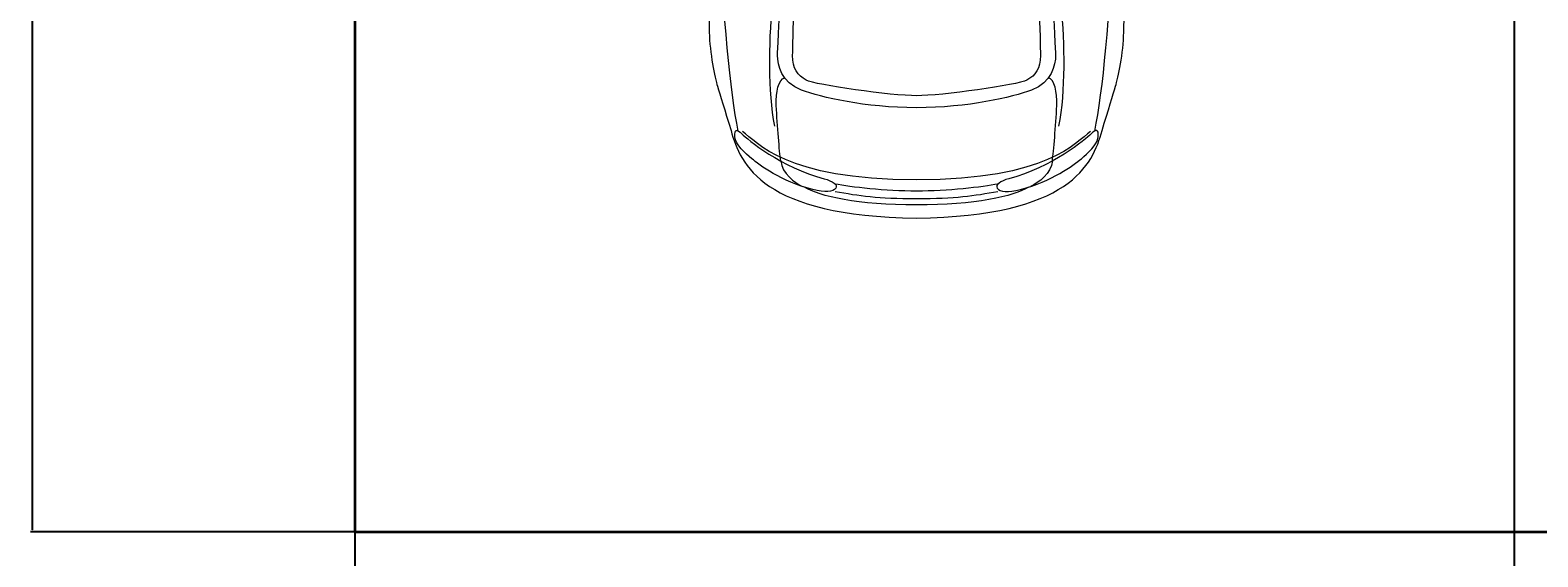
# Model space of a CAD drawing. Units: inches. Extents: x 1911 to 3278, y 2022 to 3108.
# Tile 2 of 13: x 1989 to 2120, y 2132 to 2178. Entities that reach past the tile are written whole.
import ezdxf

# ---------------------------------------------------------------- set-up
doc = ezdxf.new("R2010")
doc.units = ezdxf.units.IN
for name, color, linetype, lineweight in [('A-ANNO-DIMS', 2, 'Continuous', 18), ('A-WALL', 7, 'Continuous', 35), ('AUDI', 7, 'Continuous', 18)]:
    doc.layers.add(name, color=color, linetype=linetype, lineweight=lineweight)
doc.styles.get("Standard").update_dxf_attribs({"font": 'arial.ttf'})
doc.dimstyles.get("Standard").update_dxf_attribs({"dimtxt": 0.18, "dimasz": 0.18, "dimexe": 0.18, "dimexo": 0.0625, "dimgap": 0.09, "dimtad": 0, "dimtih": 1, "dimtoh": 1, "dimdec": 4, "dimzin": 0, "dimdsep": 46, "dimtxsty": 'Standard', "dimcen": 0.09, "dimadec": 0, "dimazin": 0, "dimtfac": 1, "dimtdec": 4, "dimtofl": 0, "dimtmove": 0, "dimatfit": 3, "dimfxl": 1, "dimtolj": 1, "dimtzin": 0, "dimarcsym": 0})

# ---------------------------------------------------------------- blocks, each defined once
blk = doc.blocks.new('*D68')
at = {"layer": 'A-ANNO-DIMS', "color": 0, "lineweight": -2, "transparency": 16777216}
for p, q in [((2016.83, 2263.81), (2016.83, 2048.12)), ((2117.83, 2263.81), (2117.83, 2048.12)), ((2017.01, 2048.3), (2067.07, 2048.3)), ((2117.65, 2048.3), (2067.6, 2048.3))]:
    blk.add_line(p, q, dxfattribs=at)
at = {"layer": 'A-ANNO-DIMS', "color": 0, "transparency": 16777216}
for points in [[(2017.01, 2048.33), (2017.01, 2048.27), (2016.83, 2048.3)], [(2117.65, 2048.33), (2117.65, 2048.27), (2117.83, 2048.3)]]:
    blk.add_solid(points, dxfattribs=at)
at = {"layer": 'Defpoints', "color": 0, "transparency": 16777216}
for p in [(2016.83, 2263.87), (2117.83, 2263.87), (2117.83, 2048.3)]:
    blk.add_point(p, dxfattribs=at)
at = {"layer": 'A-ANNO-DIMS', "color": 0, "transparency": 16777216, "insert": (2067.33, 2048.3), "char_height": 0.18, "attachment_point": 5}
blk.add_mtext('\\A1;101', dxfattribs=at)
blk = doc.blocks.new('*D69')
at = {"layer": 'A-ANNO-DIMS', "color": 0, "lineweight": -2, "transparency": 16777216}
for p, q in [((2016.77, 2263.87), (1988.55, 2263.87)), ((1988.73, 2263.69), (1988.73, 2199.06)), ((1988.73, 2134.05), (1988.73, 2198.69)), ((2016.77, 2133.87), (1988.55, 2133.87))]:
    blk.add_line(p, q, dxfattribs=at)
at = {"layer": 'A-ANNO-DIMS', "color": 0, "transparency": 16777216}
for points in [[(1988.7, 2263.69), (1988.76, 2263.69), (1988.73, 2263.87)], [(1988.7, 2134.05), (1988.76, 2134.05), (1988.73, 2133.87)]]:
    blk.add_solid(points, dxfattribs=at)
at = {"layer": 'Defpoints', "color": 0, "transparency": 16777216}
for p in [(2016.83, 2263.87), (1988.73, 2133.87), (2016.83, 2133.87)]:
    blk.add_point(p, dxfattribs=at)
at = {"layer": 'A-ANNO-DIMS', "color": 0, "transparency": 16777216, "insert": (1988.73, 2198.87), "char_height": 0.18, "attachment_point": 5}
blk.add_mtext('\\A1;130', dxfattribs=at)
blk = doc.blocks.new('*D70')
at = {"layer": 'A-ANNO-DIMS', "color": 0, "lineweight": -2, "transparency": 16777216}
for p, q in [((2134.1, 2181.81), (2134.1, 2048.12)), ((2016.83, 2133.81), (2016.83, 2048.12)), ((2017.01, 2048.3), (2075.01, 2048.3)), ((2133.92, 2048.3), (2075.92, 2048.3))]:
    blk.add_line(p, q, dxfattribs=at)
at = {"layer": 'A-ANNO-DIMS', "color": 0, "transparency": 16777216}
for points in [[(2017.01, 2048.33), (2017.01, 2048.27), (2016.83, 2048.3)], [(2133.92, 2048.33), (2133.92, 2048.27), (2134.1, 2048.3)]]:
    blk.add_solid(points, dxfattribs=at)
at = {"layer": 'Defpoints', "color": 0, "transparency": 16777216}
for p in [(2134.1, 2181.87), (2016.83, 2133.87), (2134.1, 2048.3)]:
    blk.add_point(p, dxfattribs=at)
at = {"layer": 'A-ANNO-DIMS', "color": 0, "transparency": 16777216, "insert": (2075.47, 2048.3), "char_height": 0.18, "attachment_point": 5}
blk.add_mtext('\\A1;117.27', dxfattribs=at)

msp = doc.modelspace()

# ---------------------------------------------------------------- linework, layer by layer
at = {"layer": 'A-WALL'}
for p, q in [((2016.8344, 2620.8733), (2016.8344, 2133.8733)), ((2016.8344, 2620.8733), (2016.8344, 2133.8733)), ((2016.8344, 2133.8733), (2126.8344, 2133.8733))]:
    msp.add_line(p, q, dxfattribs=at)
at = {"layer": 'AUDI'}
for points, knots in [([(2065.7636, 2161.2036), (2052.3657, 2161.35), (2050.4204, 2165.8553), (2049.5983, 2168.8238), (2049.5983, 2168.8238), (2049.0621, 2170.5764), (2048.6333, 2171.9712), (2048.4187, 2172.6866), (2048.4187, 2172.6866), (2048.2042, 2173.4019), (2047.7397, 2175.5836), (2047.7038, 2177.4077), (2047.7038, 2177.4077), (2047.6679, 2179.2318), (2047.491, 2190.1075), (2047.491, 2193.1091), (2047.491, 2193.1091), (2047.491, 2196.1105), (2047.491, 2210.1722), (2047.491, 2212.1725), (2047.491, 2212.1725), (2047.491, 2214.1727), (2047.9184, 2222.1512), (2047.9184, 2224.6905), (2047.9184, 2224.6905), (2047.9184, 2227.23), (2047.491, 2230.416), (2047.491, 2231.7362), (2047.491, 2231.7362), (2047.491, 2233.0566), (2047.7395, 2240.034), (2047.8468, 2241.572), (2047.8468, 2241.572), (2047.9542, 2243.11), (2048.5301, 2243.9822), (2049.0266, 2245.0771), (2049.0266, 2245.0771), (2050.9569, 2249.333), (2055.8898, 2251.6577), (2056.426, 2252.0154), (2056.426, 2252.0154), (2056.9622, 2252.3732), (2057.5315, 2252.5675), (2058.2133, 2252.5675), (2058.2133, 2252.5675), (2058.8952, 2252.5675), (2059.0712, 2252.2302), (2059.3573, 2252.3017), (2059.3573, 2252.3017), (2059.6432, 2252.3732), (2060.3558, 2252.5675), (2061.1448, 2252.5675), (2061.1448, 2252.5675), (2061.9338, 2252.5675), (2065.7636, 2252.5675), (2065.7636, 2252.5675), (2065.7636, 2252.5675), (2065.7636, 2252.5675), (2069.5936, 2252.5675), (2070.3825, 2252.5675), (2070.3825, 2252.5675), (2071.1717, 2252.5675), (2071.8841, 2252.3732), (2072.1701, 2252.3017), (2072.1701, 2252.3017), (2072.4561, 2252.2302), (2072.6322, 2252.5675), (2073.314, 2252.5675), (2073.314, 2252.5675), (2073.9959, 2252.5675), (2074.5651, 2252.3732), (2075.1013, 2252.0154), (2075.1013, 2252.0154), (2075.6375, 2251.6577), (2080.5704, 2249.333), (2082.5007, 2245.0771), (2082.5007, 2245.0771), (2082.9972, 2243.9822), (2083.5731, 2243.1099), (2083.6805, 2241.572), (2083.6805, 2241.572), (2083.7879, 2240.0341), (2084.0364, 2233.0565), (2084.0364, 2231.7362), (2084.0364, 2231.7362), (2084.0364, 2230.4161), (2083.609, 2227.23), (2083.609, 2224.6905), (2083.609, 2224.6905), (2083.609, 2222.1512), (2084.0364, 2214.1727), (2084.0364, 2212.1725), (2084.0364, 2212.1725), (2084.0364, 2210.1722), (2084.0364, 2196.1105), (2084.0364, 2193.1091), (2084.0364, 2193.1091), (2084.0364, 2190.1075), (2083.8594, 2179.2318), (2083.8235, 2177.4077), (2083.8235, 2177.4077), (2083.7877, 2175.5836), (2083.3232, 2173.4019), (2083.1086, 2172.6866), (2083.1086, 2172.6866), (2082.8941, 2171.9712), (2082.4652, 2170.5764), (2081.9291, 2168.8238), (2081.9291, 2168.8238), (2081.107, 2165.8553), (2079.1616, 2161.35), (2065.7636, 2161.2036)], [0, 0, 0, 0, 0.03571429, 0.03571429, 0.03571429, 0.0357143, 0.07142857, 0.07142857, 0.07142857, 0.07142858, 0.10714286, 0.10714286, 0.10714286, 0.10714287, 0.14285714, 0.14285714, 0.14285714, 0.14285715, 0.17857143, 0.17857143, 0.17857143, 0.17857144, 0.21428571, 0.21428571, 0.21428571, 0.21428572, 0.25, 0.25, 0.25, 0.25000001, 0.28571429, 0.28571429, 0.28571429, 0.2857143, 0.32142857, 0.32142857, 0.32142857, 0.32142858, 0.35714286, 0.35714286, 0.35714286, 0.35714287, 0.39285714, 0.39285714, 0.39285714, 0.39285715, 0.42857143, 0.42857143, 0.42857143, 0.42857144, 0.46428571, 0.46428571, 0.46428571, 0.46428572, 0.5, 0.5, 0.5, 0.50000001, 0.53571429, 0.53571429, 0.53571429, 0.5357143, 0.57142857, 0.57142857, 0.57142857, 0.57142858, 0.60714286, 0.60714286, 0.60714286, 0.60714287, 0.64285714, 0.64285714, 0.64285714, 0.64285715, 0.67857143, 0.67857143, 0.67857143, 0.67857144, 0.71428571, 0.71428571, 0.71428571, 0.71428572, 0.75, 0.75, 0.75, 0.75000001, 0.78571429, 0.78571429, 0.78571429, 0.7857143, 0.82142857, 0.82142857, 0.82142857, 0.82142858, 0.85714286, 0.85714286, 0.85714286, 0.85714287, 0.89285714, 0.89285714, 0.89285714, 0.89285715, 0.92857143, 0.92857143, 0.92857143, 0.92857144, 0.96428571, 0.96428571, 0.96428571, 0.96428572, 1, 1, 1, 1]), ([(2050.2266, 2168.7846), (2049.5535, 2172.1525), (2048.8368, 2178.9728), (2048.7144, 2186.0758), (2048.7144, 2186.0758), (2048.5919, 2193.1787), (2048.2861, 2220.4882), (2048.4696, 2226.2439), (2048.4696, 2226.2439), (2048.6532, 2231.9997), (2048.7559, 2239.2607), (2049.7755, 2244.2027)], [0, 0, 0, 0, 0.33333333, 0.33333333, 0.33333333, 0.33333334, 0.66666667, 0.66666667, 0.66666667, 0.66666668, 1, 1, 1, 1]), ([(2081.3007, 2168.7846), (2081.9739, 2172.1525), (2082.6906, 2178.9728), (2082.813, 2186.0758), (2082.813, 2186.0758), (2082.9355, 2193.1787), (2083.2413, 2220.4882), (2083.0577, 2226.2439), (2083.0577, 2226.2439), (2082.8742, 2231.9997), (2082.7714, 2239.2607), (2081.7518, 2244.2027)], [0, 0, 0, 0, 0.33333333, 0.33333333, 0.33333333, 0.33333334, 0.66666667, 0.66666667, 0.66666667, 0.66666668, 1, 1, 1, 1]), ([(2054.0235, 2212.6996), (2054.5037, 2204.0341), (2054.0518, 2190.4068), (2053.9475, 2187.6412), (2053.9475, 2187.6412), (2053.8432, 2184.8757), (2052.1504, 2175.4823), (2053.3909, 2169.197)], [0, 0, 0, 0, 0.5, 0.5, 0.5, 0.50000001, 1, 1, 1, 1]), ([(2077.5039, 2212.6996), (2077.0237, 2204.0341), (2077.4756, 2190.4068), (2077.5799, 2187.6412), (2077.5799, 2187.6412), (2077.6842, 2184.8757), (2079.3769, 2175.4823), (2078.1365, 2169.197)], [0, 0, 0, 0, 0.5, 0.5, 0.5, 0.50000001, 1, 1, 1, 1]), ([(2065.7636, 2170.8144), (2070.2681, 2170.8144), (2074.0546, 2171.7187), (2075.793, 2172.345), (2075.793, 2172.345), (2077.5314, 2172.9711), (2077.8792, 2174.5714), (2077.8792, 2175.3715), (2077.8792, 2175.3715), (2077.8792, 2176.1716), (2077.3227, 2184.9729), (2077.2533, 2185.5992), (2077.2533, 2185.5992), (2077.1838, 2186.2254), (2077.2184, 2186.782), (2075.8625, 2186.434), (2075.8625, 2186.434), (2074.5064, 2186.0861), (2067.4483, 2185.2513), (2065.7636, 2185.2513), (2065.7636, 2185.2513), (2064.0791, 2185.2513), (2057.0209, 2186.0861), (2055.6649, 2186.434), (2055.6649, 2186.434), (2054.3089, 2186.782), (2054.3435, 2186.2254), (2054.274, 2185.5992), (2054.274, 2185.5992), (2054.2046, 2184.9729), (2053.6482, 2176.1716), (2053.6482, 2175.3715), (2053.6482, 2175.3715), (2053.6482, 2174.5714), (2053.996, 2172.9711), (2055.7344, 2172.345), (2055.7344, 2172.345), (2057.4727, 2171.7187), (2061.2592, 2170.8144), (2065.7636, 2170.8144)], [0, 0, 0, 0, 0.1, 0.1, 0.1, 0.10000001, 0.2, 0.2, 0.2, 0.20000001, 0.3, 0.3, 0.3, 0.30000001, 0.4, 0.4, 0.4, 0.40000001, 0.5, 0.5, 0.5, 0.50000001, 0.6, 0.6, 0.6, 0.60000001, 0.7, 0.7, 0.7, 0.70000001, 0.8, 0.8, 0.8, 0.80000001, 0.9, 0.9, 0.9, 0.90000001, 1, 1, 1, 1]), ([(2065.7636, 2170.8144), (2070.2681, 2170.8144), (2074.0546, 2171.7187), (2075.793, 2172.345), (2075.793, 2172.345), (2077.5314, 2172.9711), (2077.8792, 2174.5714), (2077.8792, 2175.3715), (2077.8792, 2175.3715), (2077.8792, 2176.1716), (2077.3227, 2184.9729), (2077.2533, 2185.5992), (2077.2533, 2185.5992), (2077.1838, 2186.2254), (2077.2184, 2186.782), (2075.8625, 2186.434), (2075.8625, 2186.434), (2074.5064, 2186.0861), (2067.4483, 2185.2513), (2065.7636, 2185.2513), (2065.7636, 2185.2513), (2064.0791, 2185.2513), (2057.0209, 2186.0861), (2055.6649, 2186.434), (2055.6649, 2186.434), (2054.3089, 2186.782), (2054.3435, 2186.2254), (2054.274, 2185.5992), (2054.274, 2185.5992), (2054.2046, 2184.9729), (2053.6482, 2176.1716), (2053.6482, 2175.3715), (2053.6482, 2175.3715), (2053.6482, 2174.5714), (2053.996, 2172.9711), (2055.7344, 2172.345), (2055.7344, 2172.345), (2057.4727, 2171.7187), (2061.2592, 2170.8144), (2065.7636, 2170.8144)], [0, 0, 0, 0, 0.1, 0.1, 0.1, 0.10000001, 0.2, 0.2, 0.2, 0.20000001, 0.3, 0.3, 0.3, 0.30000001, 0.4, 0.4, 0.4, 0.40000001, 0.5, 0.5, 0.5, 0.50000001, 0.6, 0.6, 0.6, 0.60000001, 0.7, 0.7, 0.7, 0.70000001, 0.8, 0.8, 0.8, 0.80000001, 0.9, 0.9, 0.9, 0.90000001, 1, 1, 1, 1]), ([(2065.7636, 2171.8557), (2067.9003, 2171.8557), (2074.6107, 2172.7972), (2075.3757, 2173.2147), (2075.3757, 2173.2147), (2076.1407, 2173.6321), (2076.5579, 2174.2235), (2076.5579, 2175.3715), (2076.5579, 2175.3715), (2076.5579, 2176.5194), (2076.3491, 2182.9553), (2076.2797, 2183.9989), (2076.2797, 2183.9989), (2076.2102, 2185.0426), (2075.2715, 2185.147), (2074.3327, 2185.0078), (2074.3327, 2185.0078), (2073.3938, 2184.8686), (2070.0908, 2184.0686), (2065.7636, 2184.0686), (2065.7636, 2184.0686), (2061.4365, 2184.0686), (2058.1335, 2184.8686), (2057.1947, 2185.0078), (2057.1947, 2185.0078), (2056.2559, 2185.147), (2055.3171, 2185.0426), (2055.2476, 2183.9989), (2055.2476, 2183.9989), (2055.1782, 2182.9553), (2054.9693, 2176.5194), (2054.9693, 2175.3715), (2054.9693, 2175.3715), (2054.9693, 2174.2235), (2055.3866, 2173.6321), (2056.1516, 2173.2147), (2056.1516, 2173.2147), (2056.9166, 2172.7973), (2063.627, 2171.8557), (2065.7636, 2171.8557)], [0, 0, 0, 0, 0.1, 0.1, 0.1, 0.10000001, 0.2, 0.2, 0.2, 0.20000001, 0.3, 0.3, 0.3, 0.30000001, 0.4, 0.4, 0.4, 0.40000001, 0.5, 0.5, 0.5, 0.50000001, 0.6, 0.6, 0.6, 0.60000001, 0.7, 0.7, 0.7, 0.70000001, 0.8, 0.8, 0.8, 0.80000001, 0.9, 0.9, 0.9, 0.90000001, 1, 1, 1, 1]), ([(2053.9269, 2166.1743), (2053.8242, 2167.0325), (2053.6211, 2169.2283), (2053.5439, 2171.0057), (2053.5439, 2171.0057), (2053.4917, 2172.2058), (2053.7493, 2173.2756), (2054.2724, 2173.419)], [0, 0, 0, 0, 0.5, 0.5, 0.5, 0.50000001, 1, 1, 1, 1]), ([(2077.6004, 2166.1743), (2077.7031, 2167.0325), (2077.9062, 2169.2283), (2077.9835, 2171.0057), (2077.9835, 2171.0057), (2078.0356, 2172.2058), (2077.7781, 2173.2756), (2077.2549, 2173.419)], [0, 0, 0, 0, 0.5, 0.5, 0.5, 0.50000001, 1, 1, 1, 1]), ([(2057.7207, 2164.6266), (2054.0062, 2165.5874), (2050.9978, 2168.0912), (2050.5338, 2168.5416), (2050.5338, 2168.5416), (2050.1256, 2168.9381), (2049.8748, 2168.9816), (2049.9385, 2168.2832), (2049.9385, 2168.2832), (2050.0015, 2167.5942), (2050.8702, 2166.818), (2051.4034, 2166.3758), (2051.4034, 2166.3758), (2052.0844, 2165.8108), (2053.954, 2164.4005), (2056.7162, 2163.6972), (2056.7162, 2163.6972), (2057.7708, 2163.3956), (2058.5242, 2163.4962), (2058.7251, 2163.7976), (2058.7251, 2163.7976), (2058.926, 2164.0991), (2058.4584, 2164.4349), (2057.7207, 2164.6266)], [0, 0, 0, 0, 0.16666667, 0.16666667, 0.16666667, 0.16666668, 0.33333333, 0.33333333, 0.33333333, 0.33333334, 0.5, 0.5, 0.5, 0.50000001, 0.66666667, 0.66666667, 0.66666667, 0.66666668, 0.83333333, 0.83333333, 0.83333333, 0.83333334, 1, 1, 1, 1]), ([(2073.8066, 2164.6266), (2077.5212, 2165.5874), (2080.5297, 2168.0912), (2080.9935, 2168.5416), (2080.9935, 2168.5416), (2081.4018, 2168.9381), (2081.6526, 2168.9816), (2081.5888, 2168.2832), (2081.5888, 2168.2832), (2081.5259, 2167.5942), (2080.6572, 2166.818), (2080.1241, 2166.3758), (2080.1241, 2166.3758), (2079.4429, 2165.8108), (2077.5734, 2164.4005), (2074.8112, 2163.6972), (2074.8112, 2163.6972), (2073.7565, 2163.3956), (2073.0031, 2163.4962), (2072.8023, 2163.7976), (2072.8023, 2163.7976), (2072.6014, 2164.0991), (2073.069, 2164.4349), (2073.8066, 2164.6266)], [0, 0, 0, 0, 0.16666667, 0.16666667, 0.16666667, 0.16666668, 0.33333333, 0.33333333, 0.33333333, 0.33333334, 0.5, 0.5, 0.5, 0.50000001, 0.66666667, 0.66666667, 0.66666667, 0.66666668, 0.83333333, 0.83333333, 0.83333333, 0.83333334, 1, 1, 1, 1]), ([(2080.9295, 2168.7348), (2079.6002, 2167.8225), (2077.3262, 2164.535), (2065.7636, 2164.535), (2065.7636, 2164.535), (2054.2011, 2164.535), (2051.9271, 2167.8225), (2050.5978, 2168.7348)], [0, 0, 0, 0, 0.5, 0.5, 0.5, 0.50000001, 1, 1, 1, 1]), ([(2075.5194, 2163.8985), (2074.2284, 2163.0742), (2070.8591, 2162.3437), (2065.7636, 2162.3437), (2065.7636, 2162.3437), (2060.6682, 2162.3437), (2057.299, 2163.0742), (2056.008, 2163.8985)], [0, 0, 0, 0, 0.5, 0.5, 0.5, 0.50000001, 1, 1, 1, 1]), ([(2072.8581, 2164.1644), (2071.5163, 2163.9089), (2068.46, 2163.5436), (2065.7636, 2163.5436), (2065.7636, 2163.5436), (2063.0673, 2163.5436), (2060.011, 2163.9089), (2058.6693, 2164.1644)], [0, 0, 0, 0, 0.5, 0.5, 0.5, 0.50000001, 1, 1, 1, 1]), ([(2072.8581, 2163.4915), (2070.7861, 2163.1263), (2069.138, 2162.8654), (2065.7636, 2162.8654), (2065.7636, 2162.8654), (2062.3893, 2162.8654), (2060.7412, 2163.1263), (2058.6693, 2163.4915)], [0, 0, 0, 0, 0.5, 0.5, 0.5, 0.50000001, 1, 1, 1, 1])]:
    msp.add_open_spline(points, degree=3, knots=knots, dxfattribs=at)
for points in [[(2053.9269, 2166.1743), (2054.0441, 2165.0752), (2055.122, 2164.2913), (2055.8232, 2163.9578)], [(2077.6004, 2166.1743), (2077.4833, 2165.0752), (2076.4054, 2164.2913), (2075.7042, 2163.9578)]]:
    msp.add_open_spline(points, degree=3, dxfattribs=at)

# ---------------------------------------------------------------- dimensions: what is measured, and where the dimension line sits
at = {"layer": 'A-ANNO-DIMS'}
dim = msp.add_linear_dim(base=(1988.7344, 2133.8733), p1=(2016.8344, 2263.8733), p2=(2016.8344, 2133.8733), angle=90, dimstyle='Standard', override={"dimdec": 0, "dimlfac": 1, "dimrnd": 0, "dimzin": 0, "dimdsep": 46, "dimlunit": 2}, dxfattribs=at)
dim.commit()
dim.dimension.update_dxf_attribs({"geometry": '*D69', "text_midpoint": (1988.7344, 2198.8733)})
for base, p1, p2, override, picture, middle in [((2117.8344, 2048.3043), (2016.8344, 2263.8733), (2117.8344, 2263.8733), {"dimdec": 0, "dimlfac": 1, "dimrnd": 0, "dimzin": 0, "dimdsep": 46, "dimlunit": 2}, '*D68', (2067.3344, 2048.3043)), ((2134.1034, 2048.3043), (2016.8344, 2133.8733), (2134.1034, 2181.8733), {"dimdec": 2, "dimlfac": 1, "dimrnd": 0, "dimzin": 0, "dimdsep": 46, "dimlunit": 2}, '*D70', (2075.4689, 2048.3043))]:
    dim = msp.add_linear_dim(base=base, p1=p1, p2=p2, dimstyle='Standard', override=override, dxfattribs=at)
    dim.commit()
    dim.dimension.update_dxf_attribs({"geometry": picture, "text_midpoint": middle})

doc.saveas('drawing.dxf')
